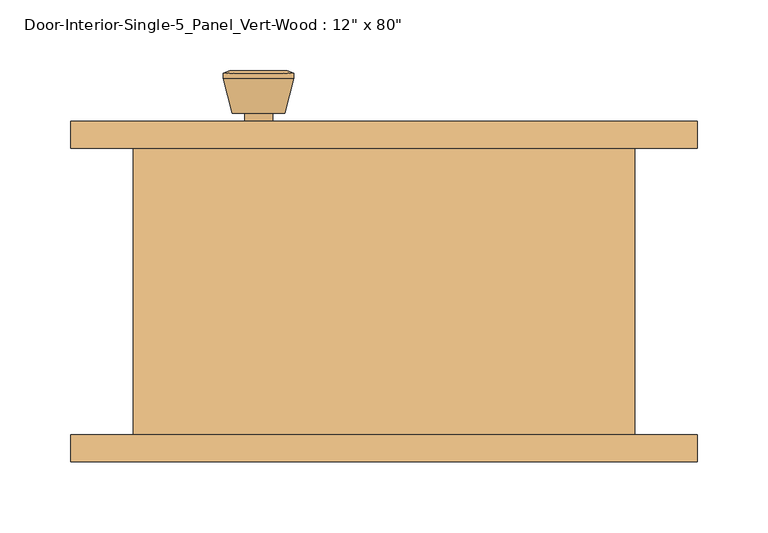
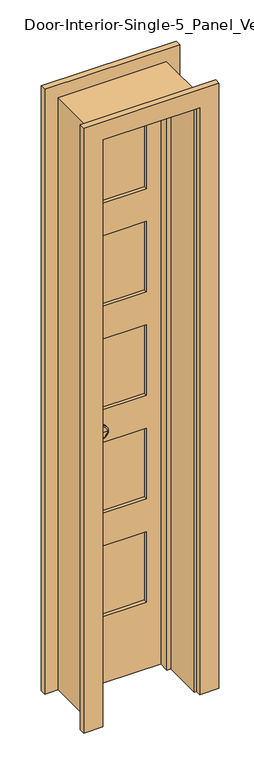
"""IFC4 building model written with IfcOpenShell, lengths in millimetres: door geometry."""

from ifc_helpers import new_model, si_unit, point, frame, frame_2d, origin, place, context, project, spatial, polyline, circle_curve, trimmed, segment, composite_curve, outline, extrude, faceted_brep, source, transform, mapped, element, save
from ifc_brep_helpers import plane_surface, cylinder_surface, revolved_surface, advanced_brep


def door_5a382651(model_context):
    return source(origin(), model_context, "Body", "SolidModel", [
        advanced_brep(
        [(-88.9, 57.5, 914.4), (-78.9, 57.5, 914.4), (-98.9, 57.5, 914.4), (-68.4241324, 8.5, 914.4), (-88.9, 8.5, 914.4), (-109.3758676, 8.5, 914.4), (-63.9, 10.3278681, 914.4), (-113.9, 10.3278681, 914.4), (-63.9, 13.7915463, 914.4), (-113.9, 13.7915463, 914.4), (-70.263764, 38.5, 914.4), (-107.536236, 38.5, 914.4), (-78.9, 38.5, 914.4), (-98.9, 38.5, 914.4)],
        [
            (0, 1),
            (1, 2, circle_curve(frame((-88.9, 57.5, 914.4), z_axis=(0.0, 1.0, 0.0), x_axis=(-1.0, 0.0, 0.0)), 10.0)),
            (2, 0),
            (2, 1, circle_curve(frame((-88.9, 57.5, 914.4), z_axis=(0.0, 1.0, 0.0), x_axis=(-1.0, 0.0, 0.0)), 10.0)),
            (3, 4),
            (4, 5),
            (5, 3, circle_curve(frame((-88.9, 8.5, 914.4), z_axis=(0.0, -1.0, 0.0), x_axis=(-1.0, 0.0, 0.0)), 20.4758676)),
            (3, 5, circle_curve(frame((-88.9, 8.5, 914.4), z_axis=(0.0, -1.0, 0.0), x_axis=(-1.0, 0.0, 0.0)), 20.4758676)),
            (6, 3),
            (5, 7),
            (7, 6, circle_curve(frame((-88.9, 10.3278681, 914.4), z_axis=(0.0, -1.0, 0.0), x_axis=(-1.0, 0.0, 0.0)), 25.0)),
            (6, 7, circle_curve(frame((-88.9, 10.3278681, 914.4), z_axis=(0.0, -1.0, 0.0), x_axis=(-1.0, 0.0, 0.0)), 25.0)),
            (8, 6),
            (7, 9),
            (9, 8, circle_curve(frame((-88.9, 13.7915463, 914.4), z_axis=(0.0, -1.0, 0.0), x_axis=(-1.0, 0.0, 0.0)), 25.0)),
            (8, 9, circle_curve(frame((-88.9, 13.7915463, 914.4), z_axis=(0.0, -1.0, 0.0), x_axis=(-1.0, 0.0, 0.0)), 25.0)),
            (10, 8),
            (9, 11),
            (11, 10, circle_curve(frame((-88.9, 38.5, 914.4), z_axis=(0.0, -1.0, 0.0), x_axis=(-1.0, 0.0, 0.0)), 18.636236)),
            (10, 11, circle_curve(frame((-88.9, 38.5, 914.4), z_axis=(0.0, -1.0, 0.0), x_axis=(-1.0, 0.0, 0.0)), 18.636236)),
            (12, 10),
            (11, 13),
            (13, 12, circle_curve(frame((-88.9, 38.5, 914.4), z_axis=(0.0, -1.0, 0.0), x_axis=(-1.0, 0.0, 0.0)), 10.0)),
            (12, 13, circle_curve(frame((-88.9, 38.5, 914.4), z_axis=(0.0, -1.0, 0.0), x_axis=(-1.0, 0.0, 0.0)), 10.0)),
            (1, 12),
            (13, 2),
        ],
        [
            plane_surface(frame((-88.9, 57.5, 914.4), z_axis=(0.0, 1.0, 0.0), x_axis=(-1.0, 0.0, 0.0))),
            plane_surface(frame((-88.9, 8.5, 914.4), z_axis=(0.0, -1.0, 0.0), x_axis=(-1.0, 0.0, 0.0))),
            revolved_surface(polyline([(-109.3758676, 8.5, 914.4), (-113.9, 10.3278681, 914.4)]), (-88.9, 57.5, 914.4), (0.0, 1.0, 0.0)),
            cylinder_surface(frame((-88.9, 57.5, 914.4), z_axis=(0.0, 1.0, 0.0), x_axis=(-1.0, 0.0, 0.0)), 25.0),
            revolved_surface(polyline([(-113.9, 13.7915463, 914.4), (-107.536236, 38.5, 914.4)]), (-88.9, 57.5, 914.4), (0.0, 1.0, 0.0)),
            plane_surface(frame((-88.9, 38.5, 914.4), z_axis=(0.0, 1.0, 0.0), x_axis=(-1.0, 0.0, 0.0))),
            cylinder_surface(frame((-88.9, 57.5, 914.4), z_axis=(0.0, 1.0, 0.0), x_axis=(-1.0, 0.0, 0.0)), 10.0),
        ],
        [
            (0, [[1, 2, 3]]),
            (0, [[-3, 4, -1]]),
            (1, [[5, 6, 7]]),
            (1, [[-6, -5, 8]]),
            (2, [[9, -7, 10, 11]]),
            (2, [[-10, -8, -9, 12]]),
            (3, [[13, -11, 14, 15]]),
            (3, [[-14, -12, -13, 16]]),
            (4, [[17, -15, 18, 19]]),
            (4, [[-18, -16, -17, 20]]),
            (5, [[21, -19, 22, 23]]),
            (5, [[-22, -20, -21, 24]]),
            (6, [[25, -23, 26, -2]]),
            (6, [[-26, -24, -25, -4]]),
        ],
    ),
        extrude(outline(composite_curve([segment(trimmed(circle_curve(frame_2d((914.4, -88.9)), 30.0), [point((914.4, -118.9))], [point((914.4, -58.9))], False, "CARTESIAN"), True, "CONTINUOUS"), segment(trimmed(circle_curve(frame_2d((914.4, -88.9)), 30.0), [point((914.4, -58.9))], [point((914.4, -118.9))], False, "CARTESIAN"), True, "CONTINUOUS")], self_intersect=False)), frame((0.0, 57.5, 0.0), z_axis=(0.0, 1.0, 0.0), x_axis=(0.0, 0.0, 1.0)), (0.0, 0.0, 1.0), 6.0),
        advanced_brep(
        [(-88.9, 104.425, 914.4), (-98.9, 104.425, 914.4), (-78.9, 104.425, 914.4), (-68.4241324, 153.425, 914.4), (-109.3758676, 153.425, 914.4), (-88.9, 153.425, 914.4), (-63.9, 151.5971319, 914.4), (-113.9, 151.5971319, 914.4), (-63.9, 148.1334537, 914.4), (-113.9, 148.1334537, 914.4), (-70.263764, 123.425, 914.4), (-107.536236, 123.425, 914.4), (-78.9, 123.425, 914.4), (-98.9, 123.425, 914.4)],
        [
            (0, 1),
            (1, 2, circle_curve(frame((-88.9, 104.425, 914.4), z_axis=(0.0, -1.0, 0.0), x_axis=(-1.0, 0.0, 0.0)), 10.0)),
            (2, 0),
            (2, 1, circle_curve(frame((-88.9, 104.425, 914.4), z_axis=(0.0, -1.0, 0.0), x_axis=(-1.0, 0.0, 0.0)), 10.0)),
            (3, 4, circle_curve(frame((-88.9, 153.425, 914.4), z_axis=(0.0, 1.0, 0.0), x_axis=(-1.0, 0.0, 0.0)), 20.4758676)),
            (4, 5),
            (5, 3),
            (4, 3, circle_curve(frame((-88.9, 153.425, 914.4), z_axis=(0.0, 1.0, 0.0), x_axis=(-1.0, 0.0, 0.0)), 20.4758676)),
            (6, 7, circle_curve(frame((-88.9, 151.5971319, 914.4), z_axis=(0.0, 1.0, 0.0), x_axis=(-1.0, 0.0, 0.0)), 25.0)),
            (7, 4),
            (3, 6),
            (7, 6, circle_curve(frame((-88.9, 151.5971319, 914.4), z_axis=(0.0, 1.0, 0.0), x_axis=(-1.0, 0.0, 0.0)), 25.0)),
            (8, 9, circle_curve(frame((-88.9, 148.1334537, 914.4), z_axis=(0.0, 1.0, 0.0), x_axis=(-1.0, 0.0, 0.0)), 25.0)),
            (9, 7),
            (6, 8),
            (9, 8, circle_curve(frame((-88.9, 148.1334537, 914.4), z_axis=(0.0, 1.0, 0.0), x_axis=(-1.0, 0.0, 0.0)), 25.0)),
            (10, 11, circle_curve(frame((-88.9, 123.425, 914.4), z_axis=(0.0, 1.0, 0.0), x_axis=(-1.0, 0.0, 0.0)), 18.636236)),
            (11, 9),
            (8, 10),
            (11, 10, circle_curve(frame((-88.9, 123.425, 914.4), z_axis=(0.0, 1.0, 0.0), x_axis=(-1.0, 0.0, 0.0)), 18.636236)),
            (12, 13, circle_curve(frame((-88.9, 123.425, 914.4), z_axis=(0.0, 1.0, 0.0), x_axis=(-1.0, 0.0, 0.0)), 10.0)),
            (13, 11),
            (10, 12),
            (13, 12, circle_curve(frame((-88.9, 123.425, 914.4), z_axis=(0.0, 1.0, 0.0), x_axis=(-1.0, 0.0, 0.0)), 10.0)),
            (1, 13),
            (12, 2),
        ],
        [
            plane_surface(frame((-88.9, 104.425, 914.4), z_axis=(0.0, -1.0, 0.0), x_axis=(-1.0, 0.0, 0.0))),
            plane_surface(frame((-88.9, 153.425, 914.4), z_axis=(0.0, 1.0, 0.0), x_axis=(-1.0, 0.0, 0.0))),
            revolved_surface(polyline([(-109.3758676, 153.425, 914.4), (-113.9, 151.5971319, 914.4)]), (-88.9, 104.425, 914.4), (0.0, -1.0, 0.0)),
            cylinder_surface(frame((-88.9, 104.425, 914.4), z_axis=(0.0, -1.0, 0.0), x_axis=(-1.0, 0.0, 0.0)), 25.0),
            revolved_surface(polyline([(-113.9, 148.1334537, 914.4), (-107.536236, 123.425, 914.4)]), (-88.9, 104.425, 914.4), (0.0, -1.0, 0.0)),
            plane_surface(frame((-88.9, 123.425, 914.4), z_axis=(0.0, -1.0, 0.0), x_axis=(-1.0, 0.0, 0.0))),
            cylinder_surface(frame((-88.9, 104.425, 914.4), z_axis=(0.0, -1.0, 0.0), x_axis=(-1.0, 0.0, 0.0)), 10.0),
        ],
        [
            (0, [[1, 2, 3]]),
            (0, [[-3, 4, -1]]),
            (1, [[5, 6, 7]]),
            (1, [[8, -7, -6]]),
            (2, [[9, 10, -5, 11]]),
            (2, [[12, -11, -8, -10]]),
            (3, [[13, 14, -9, 15]]),
            (3, [[16, -15, -12, -14]]),
            (4, [[17, 18, -13, 19]]),
            (4, [[20, -19, -16, -18]]),
            (5, [[21, 22, -17, 23]]),
            (5, [[24, -23, -20, -22]]),
            (6, [[-2, 25, -21, 26]]),
            (6, [[-4, -26, -24, -25]]),
        ],
    ),
        extrude(outline(composite_curve([segment(trimmed(circle_curve(frame_2d((914.4, -88.9)), 30.0), [point((914.4, -118.9))], [point((914.4, -58.9))], False, "CARTESIAN"), True, "CONTINUOUS"), segment(trimmed(circle_curve(frame_2d((914.4, -88.9)), 30.0), [point((914.4, -58.9))], [point((914.4, -118.9))], False, "CARTESIAN"), True, "CONTINUOUS")], self_intersect=False)), frame((0.0, 98.425, 0.0), z_axis=(0.0, 1.0, 0.0), x_axis=(0.0, 0.0, 1.0)), (0.0, 0.0, 1.0), 6.0),
        extrude(outline(polyline([(92.075, 75.1416667), (-92.075, 75.1416667), (-92.075, 86.7833333), (92.075, 86.7833333), (92.075, 75.1416667)])), frame((0.0, 0.0, 1668.145), z_axis=(0.0, 0.0, 1.0), x_axis=(1.0, 0.0, 0.0)), (0.0, 0.0, 1.0), 244.7925),
        extrude(outline(polyline([(92.075, 75.1416667), (-92.075, 75.1416667), (-92.075, 86.7833333), (92.075, 86.7833333), (92.075, 75.1416667)])), frame((0.0, 0.0, 1309.0525), z_axis=(0.0, 0.0, 1.0), x_axis=(1.0, 0.0, 0.0)), (0.0, 0.0, 1.0), 244.7925),
        extrude(outline(polyline([(92.075, 75.1416667), (-92.075, 75.1416667), (-92.075, 86.7833333), (92.075, 86.7833333), (92.075, 75.1416667)])), frame((0.0, 0.0, 590.8675), z_axis=(0.0, 0.0, 1.0), x_axis=(1.0, 0.0, 0.0)), (0.0, 0.0, 1.0), 244.7925),
        extrude(outline(polyline([(92.075, 75.1416667), (-92.075, 75.1416667), (-92.075, 86.7833333), (92.075, 86.7833333), (92.075, 75.1416667)])), frame((0.0, 0.0, 231.775), z_axis=(0.0, 0.0, 1.0), x_axis=(1.0, 0.0, 0.0)), (0.0, 0.0, 1.0), 244.7925),
        extrude(outline(polyline([(92.075, 75.1416667), (-92.075, 75.1416667), (-92.075, 86.7833333), (92.075, 86.7833333), (92.075, 75.1416667)])), frame((0.0, 0.0, 949.96), z_axis=(0.0, 0.0, 1.0), x_axis=(1.0, 0.0, 0.0)), (0.0, 0.0, 1.0), 244.7925),
        extrude(outline(polyline([(2032.0, -152.4), (0.0, -152.4), (0.0, 152.4), (2032.0, 152.4), (2032.0, -152.4)]), holes=[polyline([(1912.9375, -92.075), (1912.9375, 92.075), (1668.145, 92.075), (1668.145, -92.075), (1912.9375, -92.075)]), polyline([(476.5675, -92.075), (476.5675, 92.075), (231.775, 92.075), (231.775, -92.075), (476.5675, -92.075)]), polyline([(1194.7525, -92.075), (1194.7525, 92.075), (949.96, 92.075), (949.96, -92.075), (1194.7525, -92.075)]), polyline([(1553.845, -92.075), (1553.845, 92.075), (1309.0525, 92.075), (1309.0525, -92.075), (1553.845, -92.075)]), polyline([(835.66, -92.075), (835.66, 92.075), (590.8675, 92.075), (590.8675, -92.075), (835.66, -92.075)])]), frame((0.0, 63.5, 0.0), z_axis=(0.0, 1.0, 0.0), x_axis=(0.0, 0.0, 1.0)), (0.0, 0.0, 1.0), 34.925),
        faceted_brep([(177.8, 98.425, 0.0), (177.8, -104.775, 0.0), (152.4, -104.775, 0.0), (152.4, 28.575, 0.0), (139.7, 28.575, 0.0), (139.7, 63.5, 0.0), (152.4, 63.5, 0.0), (152.4, 98.425, 0.0), (177.8, 98.425, 2057.4), (177.8, -104.775, 2057.4), (-177.8, -104.775, 2057.4), (-177.8, -104.775, 0.0), (-152.4, -104.775, 0.0), (-152.4, -104.775, 2032.0), (152.4, -104.775, 2032.0), (152.4, 28.575, 2032.0), (-152.4, 28.575, 2032.0), (-152.4, 28.575, 0.0), (-139.7, 28.575, 0.0), (-139.7, 28.575, 2019.3), (139.7, 28.575, 2019.3), (139.7, 63.5, 2019.3), (-139.7, 63.5, 2019.3), (-139.7, 63.5, 0.0), (-152.4, 63.5, 0.0), (-152.4, 63.5, 2032.0), (152.4, 63.5, 2032.0), (152.4, 98.425, 2032.0), (-152.4, 98.425, 2032.0), (-152.4, 98.425, 0.0), (-177.8, 98.425, 0.0), (-177.8, 98.425, 2057.4)], [[[0, 1, 2, 3, 4, 5, 6, 7]], [[1, 0, 8, 9]], [[2, 1, 9, 10, 11, 12, 13, 14]], [[3, 2, 14, 15]], [[4, 3, 15, 16, 17, 18, 19, 20]], [[5, 4, 20, 21]], [[6, 5, 21, 22, 23, 24, 25, 26]], [[7, 6, 26, 27]], [[0, 7, 27, 28, 29, 30, 31, 8]], [[9, 8, 31, 10]], [[15, 14, 13, 16]], [[21, 20, 19, 22]], [[27, 26, 25, 28]], [[30, 29, 24, 23, 18, 17, 12, 11]], [[10, 31, 30, 11]], [[16, 13, 12, 17]], [[22, 19, 18, 23]], [[28, 25, 24, 29]]]),
        extrude(outline(polyline([(0.0, 158.75), (0.0, 222.25), (2101.85, 222.25), (2101.85, -222.25), (0.0, -222.25), (0.0, -158.75), (2038.35, -158.75), (2038.35, 158.75), (0.0, 158.75)])), frame((0.0, -123.825, 0.0), z_axis=(0.0, 1.0, 0.0), x_axis=(0.0, 0.0, 1.0)), (0.0, 0.0, 1.0), 19.05),
        extrude(outline(polyline([(0.0, 158.75), (0.0, 222.25), (2101.85, 222.25), (2101.85, -222.25), (0.0, -222.25), (0.0, -158.75), (2038.35, -158.75), (2038.35, 158.75), (0.0, 158.75)])), frame((0.0, 98.425, 0.0), z_axis=(0.0, 1.0, 0.0), x_axis=(0.0, 0.0, 1.0)), (0.0, 0.0, 1.0), 19.05),
    ])


if __name__ == "__main__":
    model = new_model("IFC4")
    model_context = context("Model", 3, world=origin())
    ifc_project = project(units=[si_unit("LENGTHUNIT", "METRE", prefix="MILLI")], contexts=[model_context])
    site = spatial("IfcSite", under=ifc_project)
    building = spatial("IfcBuilding", under=site)
    placement = place(None, origin())
    door_shape = door_5a382651(model_context)
    element("IfcDoor", 1, ObjectType="Door-Interior-Single-5_Panel_Vert-Wood : 12\" x 80\"", at=placement, inside=building, context=model_context, shape_type="MappedRepresentation", body=[
        mapped(door_shape, transform((0.0, 0.0, 0.0), x_axis=(1.0, 0.0, 0.0), y_axis=(0.0, 1.0, 0.0), z_axis=(0.0, 0.0, 1.0))),
    ])
    save(model, "model.ifc")

# Revit data of these elements
# Type "Door-Interior-Single-5_Panel_Vert-Wood : 12\" x 80\""
#   Type Mark = "9"
#   Assembly Code = "C1020300"
#   Analytic Construction = "Wooden"
#   Top Rail = 0' - 4 11/16"
#   Thickness = 0' - 1 3/8"
#   Thermal Resistance (R) = 2.5876 (h·ft²·°F)/BTU
#   Swing Angle [instance default] = 90.00°
#   Stiles = 0' - 2 3/8"
#   Rough Width = 1' - 2"
#   Rough Height = 6' - 9"
#   Intermediate Rail = 0' - 4 1/2"
#   Height = 6' - 8"
#   Width = 1' - 0"
#   Heat Transfer Coefficient (U) = 0.3865 BTU/(h·ft²·°F)
#   Bottom Rail = 0' - 9 1/8"
#   Trim Material = Cherry
#   Panel Material = Cherry
#   Frame Material = Cherry
#   Door Handle Material = Aluminum
#   Visual Light Transmittance = 0
#   Solar Heat Gain Coefficient = 0
#   Wall Closure = (empty or 0)
#   Function = (empty or 0)
# Element 1 (IfcDoor, "Door-Interior-Single-5_Panel_Vert-Wood : 12\" x 80\"")
#   Materials on its faces: "Cherry", "Aluminum"
# Materials
#   "Cherry": class "Wood", colour RGB 226 177 128, transparency 0, Description = "Prunus Serotina", Cost = 0
#   "Aluminum": class "Metal", colour RGB 247 247 247, transparency 0, Description = "Aluminum 6061", Cost = 0
